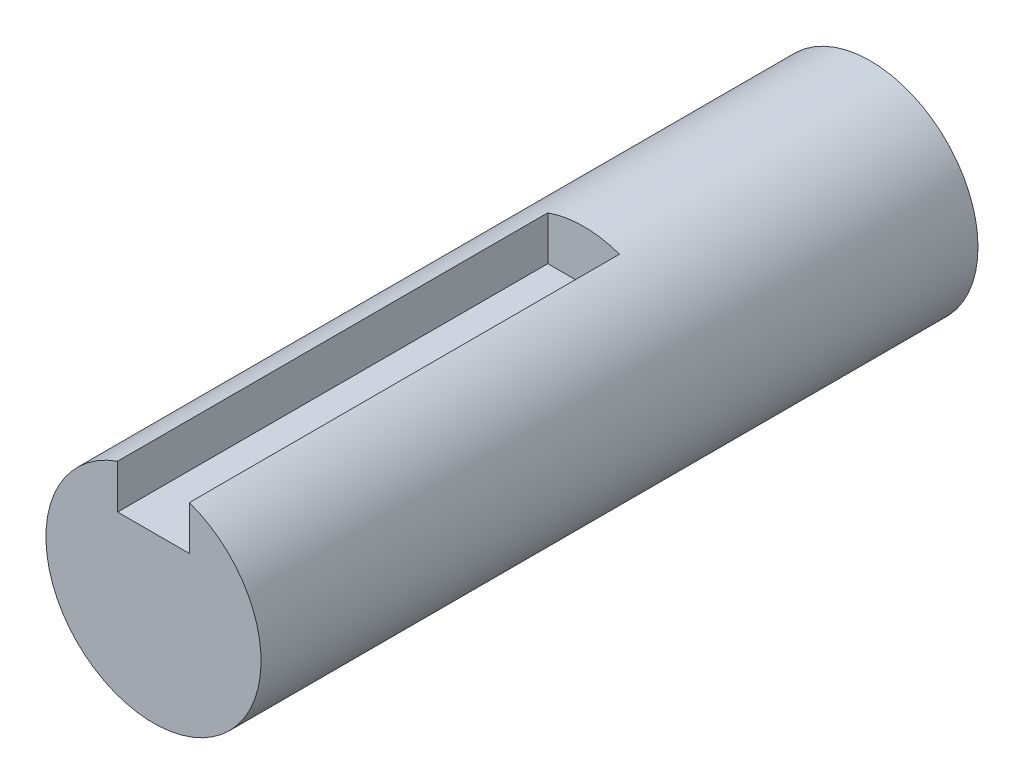
ISO-10303-21;
HEADER;
FILE_DESCRIPTION(('STEP AP214'),'2;1');
FILE_NAME('part.step','',(''),(''),'','','');
FILE_SCHEMA(('AUTOMOTIVE_DESIGN { 1 0 10303 214 1 1 1 1 }'));
ENDSEC;
DATA;
#1=APPLICATION_CONTEXT('core data for automotive mechanical design processes');
#2=APPLICATION_PROTOCOL_DEFINITION('international standard','automotive_design',2000,#1);
#3=PRODUCT_CONTEXT('',#1,'mechanical');
#4=PRODUCT('Part','Part','',(#3));
#5=PRODUCT_RELATED_PRODUCT_CATEGORY('part','',(#4));
#6=PRODUCT_DEFINITION_FORMATION('','',#4);
#7=PRODUCT_DEFINITION_CONTEXT('part definition',#1,'design');
#8=PRODUCT_DEFINITION('design','',#6,#7);
#9=PRODUCT_DEFINITION_SHAPE('','',#8);
#10=(LENGTH_UNIT() NAMED_UNIT(*) SI_UNIT(.MILLI.,.METRE.));
#11=(NAMED_UNIT(*) PLANE_ANGLE_UNIT() SI_UNIT($,.RADIAN.));
#12=(NAMED_UNIT(*) SI_UNIT($,.STERADIAN.) SOLID_ANGLE_UNIT());
#13=UNCERTAINTY_MEASURE_WITH_UNIT(LENGTH_MEASURE(1.E-05),#10,'distance_accuracy_value','');
#14=(GEOMETRIC_REPRESENTATION_CONTEXT(3) GLOBAL_UNCERTAINTY_ASSIGNED_CONTEXT((#13)) GLOBAL_UNIT_ASSIGNED_CONTEXT((#10,
#11,#12)) REPRESENTATION_CONTEXT('',''));
#15=CARTESIAN_POINT('',(0.,0.,0.));
#16=DIRECTION('',(0.,0.,1.));
#17=DIRECTION('',(1.,0.,0.));
#18=AXIS2_PLACEMENT_3D('',#15,#16,#17);
#19=CARTESIAN_POINT('',(0.,0.,100.));
#20=DIRECTION('',(0.,0.,-1.));
#21=DIRECTION('',(-1.,0.,0.));
#22=AXIS2_PLACEMENT_3D('',#19,#20,#21);
#23=CYLINDRICAL_SURFACE('',#22,15.);
#24=CARTESIAN_POINT('',(0.,0.,40.));
#25=DIRECTION('',(0.,0.,-1.));
#26=DIRECTION('',(-1.,0.,0.));
#27=AXIS2_PLACEMENT_3D('',#24,#25,#26);
#28=CIRCLE('',#27,15.);
#29=CARTESIAN_POINT('',(-5.,14.142135623731,40.));
#30=VERTEX_POINT('',#29);
#31=CARTESIAN_POINT('',(5.,14.1421356237309,40.));
#32=VERTEX_POINT('',#31);
#33=EDGE_CURVE('E11',#30,#32,#28,.T.);
#34=ORIENTED_EDGE('',*,*,#33,.T.);
#35=DIRECTION('',(0.,0.,-1.));
#36=VECTOR('',#35,1.);
#37=CARTESIAN_POINT('',(5.,14.1421356237309,100.));
#38=LINE('',#37,#36);
#39=CARTESIAN_POINT('',(5.,14.1421356237309,100.));
#40=VERTEX_POINT('',#39);
#41=EDGE_CURVE('E61',#32,#40,#38,.F.);
#42=ORIENTED_EDGE('',*,*,#41,.T.);
#43=CARTESIAN_POINT('',(0.,0.,100.));
#44=DIRECTION('',(0.,0.,1.));
#45=DIRECTION('',(1.,0.,0.));
#46=AXIS2_PLACEMENT_3D('',#43,#44,#45);
#47=CIRCLE('',#46,15.);
#48=CARTESIAN_POINT('',(-5.,14.142135623731,100.));
#49=VERTEX_POINT('',#48);
#50=EDGE_CURVE('E110',#49,#40,#47,.T.);
#51=ORIENTED_EDGE('',*,*,#50,.F.);
#52=DIRECTION('',(0.,0.,-1.));
#53=VECTOR('',#52,1.);
#54=CARTESIAN_POINT('',(-5.,14.142135623731,100.));
#55=LINE('',#54,#53);
#56=EDGE_CURVE('E52',#49,#30,#55,.T.);
#57=ORIENTED_EDGE('',*,*,#56,.T.);
#58=EDGE_LOOP('',(#34,#42,#51,#57));
#59=FACE_BOUND('',#58,.T.);
#60=CARTESIAN_POINT('',(0.,0.,0.));
#61=DIRECTION('',(0.,0.,1.));
#62=DIRECTION('',(1.,0.,0.));
#63=AXIS2_PLACEMENT_3D('',#60,#61,#62);
#64=CIRCLE('',#63,15.);
#65=CARTESIAN_POINT('',(15.,0.,0.));
#66=VERTEX_POINT('',#65);
#67=EDGE_CURVE('E106',#66,#66,#64,.T.);
#68=ORIENTED_EDGE('',*,*,#67,.T.);
#69=EDGE_LOOP('',(#68));
#70=FACE_BOUND('',#69,.T.);
#71=ADVANCED_FACE('F39',(#59,#70),#23,.T.);
#72=CARTESIAN_POINT('',(0.,0.,100.));
#73=DIRECTION('',(0.,0.,1.));
#74=DIRECTION('',(1.,0.,0.));
#75=AXIS2_PLACEMENT_3D('',#72,#73,#74);
#76=PLANE('',#75);
#77=DIRECTION('',(0.,1.,0.));
#78=VECTOR('',#77,1.);
#79=CARTESIAN_POINT('',(5.,15.,100.));
#80=LINE('',#79,#78);
#81=CARTESIAN_POINT('',(5.,8.,100.));
#82=VERTEX_POINT('',#81);
#83=EDGE_CURVE('E97',#82,#40,#80,.T.);
#84=ORIENTED_EDGE('',*,*,#83,.F.);
#85=DIRECTION('',(1.,0.,0.));
#86=VECTOR('',#85,1.);
#87=CARTESIAN_POINT('',(5.,8.,100.));
#88=LINE('',#87,#86);
#89=CARTESIAN_POINT('',(-5.,8.,100.));
#90=VERTEX_POINT('',#89);
#91=EDGE_CURVE('E101',#90,#82,#88,.T.);
#92=ORIENTED_EDGE('',*,*,#91,.F.);
#93=DIRECTION('',(0.,-1.,0.));
#94=VECTOR('',#93,1.);
#95=CARTESIAN_POINT('',(-5.,0.,100.));
#96=LINE('',#95,#94);
#97=EDGE_CURVE('E46',#49,#90,#96,.T.);
#98=ORIENTED_EDGE('',*,*,#97,.F.);
#99=ORIENTED_EDGE('',*,*,#50,.T.);
#100=EDGE_LOOP('',(#84,#92,#98,#99));
#101=FACE_BOUND('',#100,.T.);
#102=ADVANCED_FACE('F116',(#101),#76,.T.);
#103=CARTESIAN_POINT('',(0.,0.,0.));
#104=DIRECTION('',(0.,0.,1.));
#105=DIRECTION('',(1.,0.,0.));
#106=AXIS2_PLACEMENT_3D('',#103,#104,#105);
#107=PLANE('',#106);
#108=ORIENTED_EDGE('',*,*,#67,.F.);
#109=EDGE_LOOP('',(#108));
#110=FACE_BOUND('',#109,.T.);
#111=ADVANCED_FACE('F111',(#110),#107,.F.);
#112=CARTESIAN_POINT('',(0.,0.,40.));
#113=DIRECTION('',(0.,0.,-1.));
#114=DIRECTION('',(-1.,0.,0.));
#115=AXIS2_PLACEMENT_3D('',#112,#113,#114);
#116=PLANE('',#115);
#117=DIRECTION('',(0.,-1.,0.));
#118=VECTOR('',#117,1.);
#119=CARTESIAN_POINT('',(-5.,15.,40.));
#120=LINE('',#119,#118);
#121=CARTESIAN_POINT('',(-5.,8.,40.));
#122=VERTEX_POINT('',#121);
#123=EDGE_CURVE('E79',#30,#122,#120,.T.);
#124=ORIENTED_EDGE('',*,*,#123,.T.);
#125=DIRECTION('',(1.,0.,0.));
#126=VECTOR('',#125,1.);
#127=CARTESIAN_POINT('',(5.,8.,40.));
#128=LINE('',#127,#126);
#129=CARTESIAN_POINT('',(5.,8.,40.));
#130=VERTEX_POINT('',#129);
#131=EDGE_CURVE('E85',#122,#130,#128,.T.);
#132=ORIENTED_EDGE('',*,*,#131,.T.);
#133=DIRECTION('',(0.,1.,0.));
#134=VECTOR('',#133,1.);
#135=CARTESIAN_POINT('',(5.,15.,40.));
#136=LINE('',#135,#134);
#137=EDGE_CURVE('E81',#130,#32,#136,.T.);
#138=ORIENTED_EDGE('',*,*,#137,.T.);
#139=ORIENTED_EDGE('',*,*,#33,.F.);
#140=EDGE_LOOP('',(#124,#132,#138,#139));
#141=FACE_BOUND('',#140,.T.);
#142=ADVANCED_FACE('F84',(#141),#116,.F.);
#143=CARTESIAN_POINT('',(5.,15.,40.));
#144=DIRECTION('',(1.,0.,0.));
#145=DIRECTION('',(0.,1.,0.));
#146=AXIS2_PLACEMENT_3D('',#143,#144,#145);
#147=PLANE('',#146);
#148=ORIENTED_EDGE('',*,*,#137,.F.);
#149=DIRECTION('',(0.,0.,1.));
#150=VECTOR('',#149,1.);
#151=CARTESIAN_POINT('',(5.,8.,40.));
#152=LINE('',#151,#150);
#153=EDGE_CURVE('E91',#130,#82,#152,.T.);
#154=ORIENTED_EDGE('',*,*,#153,.T.);
#155=ORIENTED_EDGE('',*,*,#83,.T.);
#156=ORIENTED_EDGE('',*,*,#41,.F.);
#157=EDGE_LOOP('',(#148,#154,#155,#156));
#158=FACE_BOUND('',#157,.T.);
#159=ADVANCED_FACE('F123',(#158),#147,.F.);
#160=CARTESIAN_POINT('',(-5.,15.,40.));
#161=DIRECTION('',(-1.,0.,0.));
#162=DIRECTION('',(0.,-1.,0.));
#163=AXIS2_PLACEMENT_3D('',#160,#161,#162);
#164=PLANE('',#163);
#165=ORIENTED_EDGE('',*,*,#97,.T.);
#166=DIRECTION('',(0.,0.,1.));
#167=VECTOR('',#166,1.);
#168=CARTESIAN_POINT('',(-5.,8.,40.));
#169=LINE('',#168,#167);
#170=EDGE_CURVE('E86',#122,#90,#169,.T.);
#171=ORIENTED_EDGE('',*,*,#170,.F.);
#172=ORIENTED_EDGE('',*,*,#123,.F.);
#173=ORIENTED_EDGE('',*,*,#56,.F.);
#174=EDGE_LOOP('',(#165,#171,#172,#173));
#175=FACE_BOUND('',#174,.T.);
#176=ADVANCED_FACE('F90',(#175),#164,.F.);
#177=CARTESIAN_POINT('',(5.,8.,40.));
#178=DIRECTION('',(0.,-1.,0.));
#179=DIRECTION('',(0.,0.,-1.));
#180=AXIS2_PLACEMENT_3D('',#177,#178,#179);
#181=PLANE('',#180);
#182=ORIENTED_EDGE('',*,*,#91,.T.);
#183=ORIENTED_EDGE('',*,*,#153,.F.);
#184=ORIENTED_EDGE('',*,*,#131,.F.);
#185=ORIENTED_EDGE('',*,*,#170,.T.);
#186=EDGE_LOOP('',(#182,#183,#184,#185));
#187=FACE_BOUND('',#186,.T.);
#188=ADVANCED_FACE('F92',(#187),#181,.F.);
#189=CLOSED_SHELL('',(#71,#102,#111,#142,#159,#176,#188));
#190=MANIFOLD_SOLID_BREP('B2',#189);
#191=ADVANCED_BREP_SHAPE_REPRESENTATION('',(#18,#190),#14);
#192=SHAPE_DEFINITION_REPRESENTATION(#9,#191);
ENDSEC;
END-ISO-10303-21;
